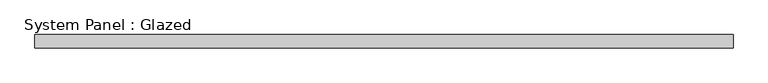
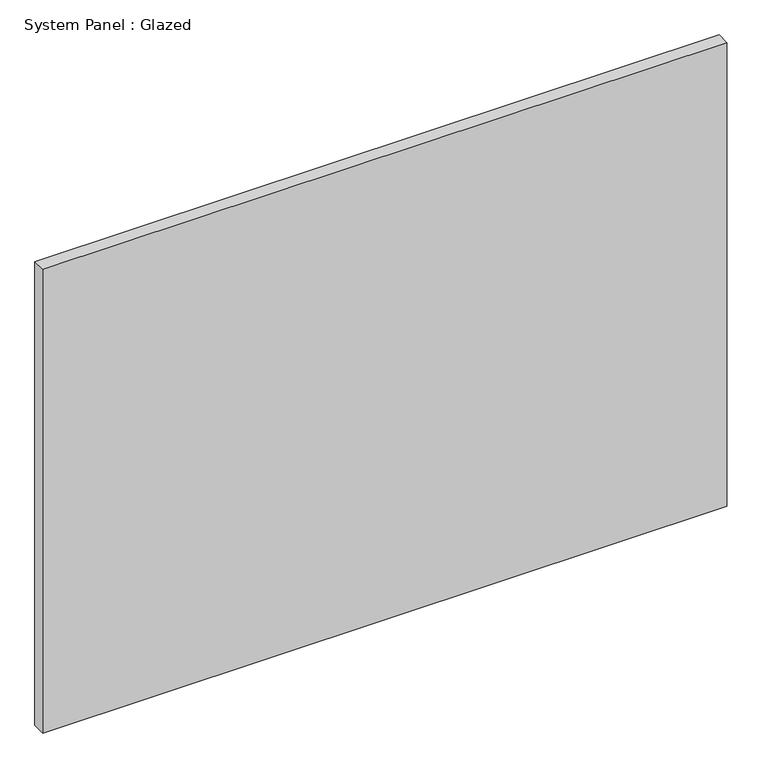
"""IFC4 building model written with IfcOpenShell, lengths in millimetres: plate geometry, System Panel : Glazed."""

from ifc_helpers import new_model, si_unit, origin, origin_with_axes, place, context, project, spatial, polyline, outline, extrude, source, transform, mapped, element, save


def system_panel_glazed_6f193a35(model_context):
    return source(origin(), model_context, "Body", "SweptSolid", [
        extrude(outline(polyline([(654.0499999, 19.05), (-654.0499999, 19.05), (-654.0499999, 44.45), (654.0499999, 44.45), (654.0499999, 19.05)])), origin_with_axes(), (0.0, 0.0, 1.0), 937.6833333),
    ])


if __name__ == "__main__":
    model = new_model("IFC4")
    model_context = context("Model", 3, world=origin())
    ifc_project = project(units=[si_unit("LENGTHUNIT", "METRE", prefix="MILLI")], contexts=[model_context])
    site = spatial("IfcSite", under=ifc_project)
    building = spatial("IfcBuilding", under=site)
    placement = place(None, origin())
    system_panel_glazed_shape = system_panel_glazed_6f193a35(model_context)
    element("IfcPlate", 1, ObjectType="System Panel : Glazed", at=placement, inside=building, context=model_context, shape_type="MappedRepresentation", body=[
        mapped(system_panel_glazed_shape, transform((0.0, 0.0, 0.0), x_axis=(1.0, 0.0, 0.0), y_axis=(0.0, 1.0, 0.0), z_axis=(0.0, 0.0, 1.0))),
    ])
    save(model, "model.ifc")

# Revit data of these elements
# Type "System Panel : Glazed"
#   Construction Type Id = "GSP4R"
#   Analytic Construction = "1/8 in Pilkington single glazing"
#   Visual Light Transmittance = 0.9
#   Solar Heat Gain Coefficient = 0.86
#   Heat Transfer Coefficient (U) = 1.18115 BTU/(h·ft²·°F)
#   Define Thermal Properties by = 1
# Element 1 (IfcPlate, "System Panel : Glazed")
#   Materials on its faces: "glass panel 223"
# Materials
#   "glass panel 223": class "Generic", colour RGB 120 120 120, transparency 0, Cost = 0
